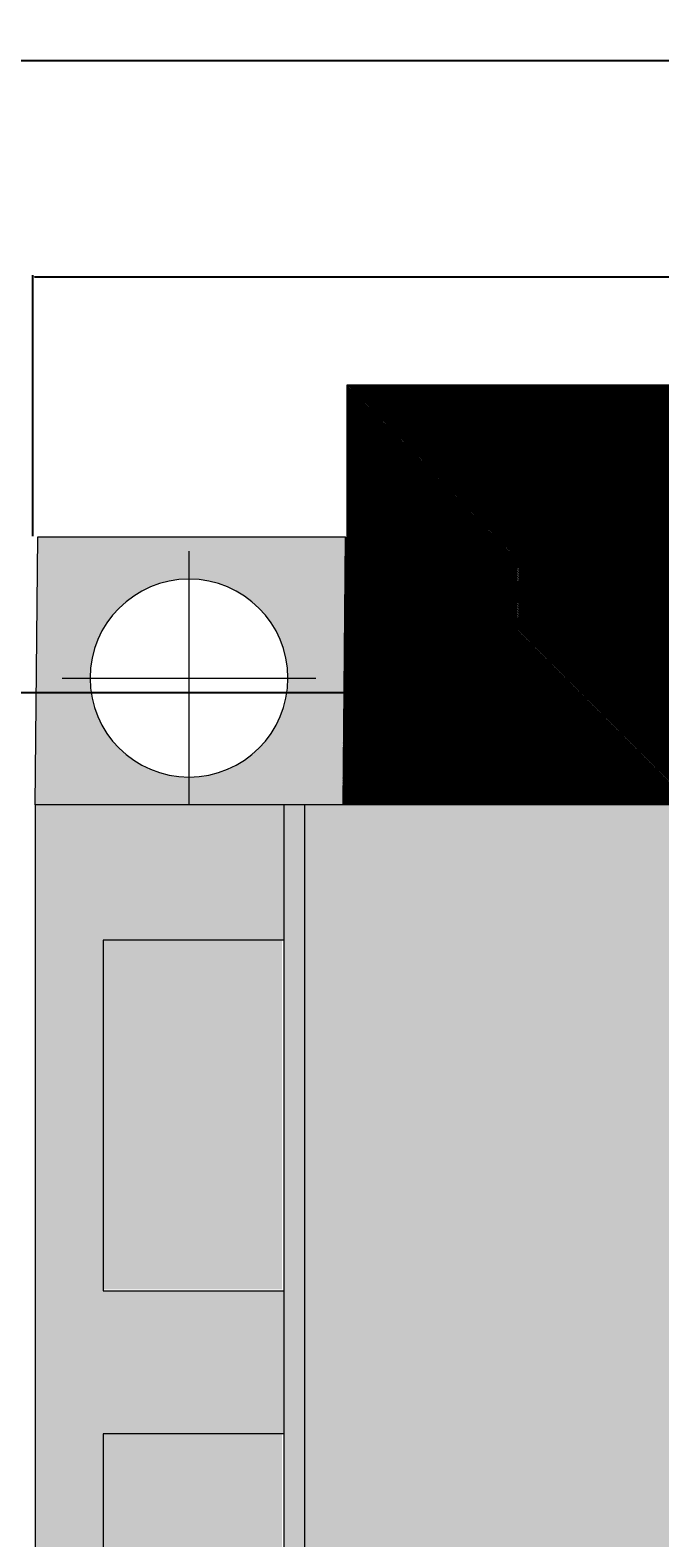
# Model space of a CAD drawing. Units: inches. Extents: x 192 to 1361, y -1362 to 367.
# Tile 7 of 23: x 293 to 361, y -616 to -454. Entities that reach past the tile are written whole.
import ezdxf

# ---------------------------------------------------------------- set-up
doc = ezdxf.new("R2010")
doc.units = ezdxf.units.IN
doc.header["$MEASUREMENT"] = 0
for name, color, linetype, lineweight in [('A-ANNO-DIMS', 2, 'Continuous', 18), ('A-FLOR', 8, 'Continuous', 18), ('furniture', 32, 'Continuous', 18)]:
    doc.layers.add(name, color=color, linetype=linetype, lineweight=lineweight)
doc.layers.add('A-FLOR-PATT', color=254, linetype='Continuous', lineweight=13, true_color=0xfeeab9)
doc.layers.add('A-FURN-PATT', color=254, linetype='Continuous', lineweight=13, true_color=0xfeeab9)
doc.styles.get("Standard").update_dxf_attribs({"font": 'arial.ttf'})
doc.dimstyles.get("Standard").update_dxf_attribs({"dimtxt": 0.18, "dimasz": 0.18, "dimexe": 0.18, "dimexo": 0.0625, "dimgap": 0.09, "dimtad": 0, "dimtih": 1, "dimtoh": 1, "dimzin": 0, "dimdsep": 46, "dimlunit": 3, "dimtxsty": 'Standard', "dimcen": 0.09, "dimadec": 0, "dimazin": 0, "dimtfac": 1, "dimtofl": 0, "dimtmove": 0, "dimatfit": 3, "dimfxl": 1, "dimtolj": 1, "dimtzin": 0, "dimarcsym": 0})

# ---------------------------------------------------------------- blocks, each defined once
blk = doc.blocks.new('A$C58D270C6')
at = {"layer": 'furniture'}
for p, q in [((14.974, 94.844), (14.974, 36)), ((16.217, 94.932), (16.217, 36)), ((9.25, 36), (9.25, 20.738)), ((1.618, 28.369), (16.881, 28.369))]:
    blk.add_line(p, q, dxfattribs=at)
for points in [[(0, 108), (77.905, 108), (77.905, 36), (0, 36)], [(4.094, 94.932), (14.974, 94.932), (14.974, 73.835), (4.094, 73.835)], [(4.094, 65.227), (14.974, 65.227), (14.974, 44.13), (4.094, 44.13)], [(18.655, 19.869), (18.499, 36), (0, 36), (0.156, 19.869)]]:
    blk.add_lwpolyline(points, close=True, dxfattribs=at)
blk.add_circle((9.25, 28.369), 5.955, dxfattribs=at)
blk = doc.blocks.new('*D24')
at = {"layer": 'A-ANNO-DIMS', "color": 0, "lineweight": -2, "transparency": 16777216}
for p, q in [((293.48, -508.38), (293.48, -480.42)), ((293.66, -480.6), (378, -480.6)), ((462.89, -480.6), (378.56, -480.6)), ((463.07, -508.38), (463.07, -480.42))]:
    blk.add_line(p, q, dxfattribs=at)
at = {"layer": 'A-ANNO-DIMS', "color": 0, "transparency": 16777216}
for points in [[(293.66, -480.57), (293.66, -480.63), (293.48, -480.6)], [(462.89, -480.57), (462.89, -480.63), (463.07, -480.6)]]:
    blk.add_solid(points, dxfattribs=at)
at = {"layer": 'Defpoints', "color": 0, "transparency": 16777216}
for p in [(463.07, -480.6), (293.48, -508.44), (463.07, -508.44)]:
    blk.add_point(p, dxfattribs=at)
at = {"layer": 'A-ANNO-DIMS', "color": 0, "transparency": 16777216, "insert": (378.28, -480.6), "char_height": 0.18, "attachment_point": 5}
blk.add_mtext('\\A1;170', dxfattribs=at)
blk = doc.blocks.new('*D48')
at = {"layer": 'A-ANNO-DIMS', "color": 0, "lineweight": -2, "transparency": 16777216}
for p, q in [((325.63, 258.53), (192.16, 258.53)), ((192.34, 258.35), (192.34, -429.22)), ((192.34, -1117.14), (192.34, -429.58)), ((395.21, -1117.32), (192.16, -1117.32))]:
    blk.add_line(p, q, dxfattribs=at)
at = {"layer": 'A-ANNO-DIMS', "color": 0, "transparency": 16777216}
for points in [[(192.31, 258.35), (192.37, 258.35), (192.34, 258.53)], [(192.31, -1117.14), (192.37, -1117.14), (192.34, -1117.32)]]:
    blk.add_solid(points, dxfattribs=at)
at = {"layer": 'Defpoints', "color": 0, "transparency": 16777216}
for p in [(325.7, 258.53), (192.34, -1117.32), (395.28, -1117.32)]:
    blk.add_point(p, dxfattribs=at)
at = {"layer": 'A-ANNO-DIMS', "color": 0, "transparency": 16777216, "insert": (192.34, -429.4), "char_height": 0.18, "attachment_point": 5}
blk.add_mtext('\\A1;1375.9', dxfattribs=at)
blk = doc.blocks.new('*D69')
at = {"layer": 'A-ANNO-DIMS', "color": 0, "lineweight": -2, "transparency": 16777216}
for p, q in [((981.75, -457.5), (192.16, -457.5)), ((192.34, -457.68), (192.34, -491.13)), ((192.34, -524.95), (192.34, -491.5)), ((980.52, -525.13), (192.16, -525.13))]:
    blk.add_line(p, q, dxfattribs=at)
at = {"layer": 'A-ANNO-DIMS', "color": 0, "transparency": 16777216}
for points in [[(192.31, -457.68), (192.37, -457.68), (192.34, -457.5)], [(192.31, -524.95), (192.37, -524.95), (192.34, -525.13)]]:
    blk.add_solid(points, dxfattribs=at)
at = {"layer": 'Defpoints', "color": 0, "transparency": 16777216}
for p in [(981.81, -457.5), (192.34, -525.13), (980.58, -525.13)]:
    blk.add_point(p, dxfattribs=at)
at = {"layer": 'A-ANNO-DIMS', "color": 0, "transparency": 16777216, "insert": (192.34, -491.31), "char_height": 0.18, "attachment_point": 5}
blk.add_mtext('\\A1;67.63', dxfattribs=at)

msp = doc.modelspace()

# ---------------------------------------------------------------- hatches: boundary and pattern name
at = {"layer": 'A-FLOR-PATT'}
h = msp.add_hatch(dxfattribs=at)
h.set_pattern_fill('ANSI31', color=256)
edge = h.paths.add_edge_path()
edge.add_line((513.1511, -492.1899), (327.1032, -492.1899))
edge.add_line((327.1032, -492.1899), (327.1032, -508.439))
edge.add_line((327.1032, -508.439), (326.9465, -508.439))
edge.add_line((326.9465, -508.439), (326.6697, -537.1419))
edge.add_line((326.6697, -537.1419), (391.8439, -537.1419))
edge.add_line((391.8439, -537.1419), (391.8439, -520.2026))
edge.add_line((391.8439, -520.2026), (393.0084, -520.2026))
edge.add_spline(control_points=[(393.2858, -517.1545), (392.9584, -517.4172), (392.3119, -517.936), (392.9583, -518.8629), (393.4257, -519.6151), (393.1386, -520.0192), (393.0084, -520.2026)], knot_values=[0, 0, 0, 0, 0.65327829, 1.2901376, 1.74045698, 2.11445126, 2.11445126, 2.11445126, 2.11445126], degree=3, periodic=0)
edge.add_line((393.0084, -520.2026), (395.1098, -520.2026))
edge.add_spline(control_points=[(395.3872, -517.1545), (395.0598, -517.4172), (394.4133, -517.936), (395.0598, -518.8629), (395.5272, -519.6151), (395.2401, -520.0192), (395.1098, -520.2026)], knot_values=[0, 0, 0, 0, 0.65327829, 1.2901376, 1.74045698, 2.11445126, 2.11445126, 2.11445126, 2.11445126], degree=3, periodic=0)
edge.add_line((395.1098, -520.2026), (397.3144, -520.2026))
edge.add_spline(control_points=[(397.5918, -517.1545), (397.2644, -517.4172), (396.6179, -517.936), (397.2643, -518.8629), (397.7317, -519.6151), (397.4446, -520.0192), (397.3144, -520.2026)], knot_values=[0, 0, 0, 0, 0.65327829, 1.2901376, 1.74045698, 2.11445126, 2.11445126, 2.11445126, 2.11445126], degree=3, periodic=0)
edge.add_line((397.3144, -520.2026), (399.2806, -520.2026))
edge.add_spline(control_points=[(399.558, -517.1545), (399.2307, -517.4172), (398.5841, -517.936), (399.2306, -518.8629), (399.698, -519.6151), (399.4109, -520.0192), (399.2806, -520.2026)], knot_values=[0, 0, 0, 0, 0.65327829, 1.2901376, 1.74045698, 2.11445126, 2.11445126, 2.11445126, 2.11445126], degree=3, periodic=0)
edge.add_line((399.2806, -520.2026), (401.664, -520.2026))
edge.add_spline(control_points=[(401.9414, -517.1545), (401.614, -517.4172), (400.9675, -517.936), (401.6139, -518.8629), (402.0814, -519.6151), (401.7943, -520.0192), (401.664, -520.2026)], knot_values=[0, 0, 0, 0, 0.65327829, 1.2901376, 1.74045698, 2.11445126, 2.11445126, 2.11445126, 2.11445126], degree=3, periodic=0)
edge.add_line((401.664, -520.2026), (403.6961, -520.2026))
edge.add_spline(control_points=[(403.9735, -517.1545), (403.6461, -517.4172), (402.9996, -517.936), (403.6461, -518.8629), (404.1135, -519.6151), (403.8264, -520.0192), (403.6961, -520.2026)], knot_values=[0, 0, 0, 0, 0.65327829, 1.2901376, 1.74045698, 2.11445126, 2.11445126, 2.11445126, 2.11445126], degree=3, periodic=0)
edge.add_line((403.6961, -520.2026), (405.6624, -520.2026))
edge.add_spline(control_points=[(405.9398, -517.1545), (405.6124, -517.4172), (404.9659, -517.936), (405.6123, -518.8629), (406.0797, -519.6151), (405.7926, -520.0192), (405.6624, -520.2026)], knot_values=[0, 0, 0, 0, 0.65327829, 1.2901376, 1.74045698, 2.11445126, 2.11445126, 2.11445126, 2.11445126], degree=3, periodic=0)
edge.add_line((405.6624, -520.2026), (408.0457, -520.2026))
edge.add_spline(control_points=[(408.3231, -517.1545), (407.9958, -517.4172), (407.3493, -517.936), (407.9957, -518.8629), (408.4631, -519.6151), (408.176, -520.0192), (408.0457, -520.2026)], knot_values=[0, 0, 0, 0, 0.65327829, 1.2901376, 1.74045698, 2.11445126, 2.11445126, 2.11445126, 2.11445126], degree=3, periodic=0)
edge.add_line((408.0457, -520.2026), (410.8462, -520.2026))
edge.add_spline(control_points=[(411.1236, -517.1545), (410.7962, -517.4172), (410.1497, -517.936), (410.7961, -518.8629), (411.2635, -519.6151), (410.9764, -520.0192), (410.8462, -520.2026)], knot_values=[0, 0, 0, 0, 0.65327829, 1.2901376, 1.74045698, 2.11445126, 2.11445126, 2.11445126, 2.11445126], degree=3, periodic=0)
edge.add_line((410.8462, -520.2026), (413.2295, -520.2026))
edge.add_spline(control_points=[(413.5069, -517.1545), (413.1795, -517.4172), (412.533, -517.936), (413.1794, -518.8629), (413.6468, -519.6151), (413.3597, -520.0192), (413.2295, -520.2026)], knot_values=[0, 0, 0, 0, 0.65327829, 1.2901376, 1.74045698, 2.11445126, 2.11445126, 2.11445126, 2.11445126], degree=3, periodic=0)
edge.add_line((413.2295, -520.2026), (415.434, -520.2026))
edge.add_spline(control_points=[(415.7114, -517.1545), (415.3841, -517.4172), (414.7376, -517.936), (415.384, -518.8629), (415.8514, -519.6151), (415.5643, -520.0192), (415.434, -520.2026)], knot_values=[0, 0, 0, 0, 0.65327829, 1.2901376, 1.74045698, 2.11445126, 2.11445126, 2.11445126, 2.11445126], degree=3, periodic=0)
edge.add_line((415.434, -520.2026), (417.5321, -520.2026))
edge.add_spline(control_points=[(417.8095, -517.1545), (417.4821, -517.4172), (416.8356, -517.936), (417.482, -518.8629), (417.9494, -519.6151), (417.6623, -520.0192), (417.5321, -520.2026)], knot_values=[0, 0, 0, 0, 0.65327829, 1.2901376, 1.74045698, 2.11445126, 2.11445126, 2.11445126, 2.11445126], degree=3, periodic=0)
edge.add_line((417.5321, -520.2026), (419.7366, -520.2026))
edge.add_spline(control_points=[(420.014, -517.1545), (419.6867, -517.4172), (419.0401, -517.936), (419.6866, -518.8629), (420.154, -519.6151), (419.8669, -520.0192), (419.7366, -520.2026)], knot_values=[0, 0, 0, 0, 0.65327829, 1.2901376, 1.74045698, 2.11445126, 2.11445126, 2.11445126, 2.11445126], degree=3, periodic=0)
edge.add_line((419.7366, -520.2026), (421.7029, -520.2026))
edge.add_spline(control_points=[(421.9803, -517.1545), (421.6529, -517.4172), (421.0064, -517.936), (421.6528, -518.8629), (422.1202, -519.6151), (421.8331, -520.0192), (421.7029, -520.2026)], knot_values=[0, 0, 0, 0, 0.65327829, 1.2901376, 1.74045698, 2.11445126, 2.11445126, 2.11445126, 2.11445126], degree=3, periodic=0)
edge.add_line((421.7029, -520.2026), (424.0863, -520.2026))
edge.add_spline(control_points=[(424.3637, -517.1545), (424.0363, -517.4172), (423.3898, -517.936), (424.0362, -518.8629), (424.5036, -519.6151), (424.2165, -520.0192), (424.0863, -520.2026)], knot_values=[0, 0, 0, 0, 0.65327829, 1.2901376, 1.74045698, 2.11445126, 2.11445126, 2.11445126, 2.11445126], degree=3, periodic=0)
edge.add_line((424.0863, -520.2026), (426.1184, -520.2026))
edge.add_spline(control_points=[(426.3958, -517.1545), (426.0684, -517.4172), (425.4219, -517.936), (426.0683, -518.8629), (426.5357, -519.6151), (426.2486, -520.0192), (426.1184, -520.2026)], knot_values=[0, 0, 0, 0, 0.65327829, 1.2901376, 1.74045698, 2.11445126, 2.11445126, 2.11445126, 2.11445126], degree=3, periodic=0)
edge.add_line((426.1184, -520.2026), (428.0846, -520.2026))
edge.add_spline(control_points=[(428.362, -517.1545), (428.0346, -517.4172), (427.3881, -517.936), (428.0346, -518.8629), (428.502, -519.6151), (428.2149, -520.0192), (428.0846, -520.2026)], knot_values=[0, 0, 0, 0, 0.65327829, 1.2901376, 1.74045698, 2.11445126, 2.11445126, 2.11445126, 2.11445126], degree=3, periodic=0)
edge.add_line((428.0846, -520.2026), (430.468, -520.2026))
edge.add_spline(control_points=[(430.7454, -517.1545), (430.418, -517.4172), (429.7715, -517.936), (430.4179, -518.8629), (430.8853, -519.6151), (430.5983, -520.0192), (430.468, -520.2026)], knot_values=[0, 0, 0, 0, 0.65327829, 1.2901376, 1.74045698, 2.11445126, 2.11445126, 2.11445126, 2.11445126], degree=3, periodic=0)
edge.add_line((430.468, -520.2026), (433.2684, -520.2026))
edge.add_spline(control_points=[(433.5458, -517.1545), (433.2184, -517.4172), (432.5719, -517.936), (433.2184, -518.8629), (433.6858, -519.6151), (433.3987, -520.0192), (433.2684, -520.2026)], knot_values=[0, 0, 0, 0, 0.65327829, 1.2901376, 1.74045698, 2.11445126, 2.11445126, 2.11445126, 2.11445126], degree=3, periodic=0)
edge.add_line((433.2684, -520.2026), (435.6517, -520.2026))
edge.add_spline(control_points=[(435.9291, -517.1545), (435.6017, -517.4172), (434.9552, -517.936), (435.6017, -518.8629), (436.0691, -519.6151), (435.782, -520.0192), (435.6517, -520.2026)], knot_values=[0, 0, 0, 0, 0.65327829, 1.2901376, 1.74045698, 2.11445126, 2.11445126, 2.11445126, 2.11445126], degree=3, periodic=0)
edge.add_line((435.6517, -520.2026), (437.8563, -520.2026))
edge.add_spline(control_points=[(438.1337, -517.1545), (437.8063, -517.4172), (437.1598, -517.936), (437.8062, -518.8629), (438.2736, -519.6151), (437.9865, -520.0192), (437.8563, -520.2026)], knot_values=[0, 0, 0, 0, 0.65327829, 1.2901376, 1.74045698, 2.11445126, 2.11445126, 2.11445126, 2.11445126], degree=3, periodic=0)
edge.add_line((437.8563, -520.2026), (439.7189, -520.2026))
edge.add_spline(control_points=[(439.9963, -517.1545), (439.669, -517.4172), (439.0225, -517.936), (439.6689, -518.8629), (440.1363, -519.6151), (439.8492, -520.0192), (439.7189, -520.2026)], knot_values=[0, 0, 0, 0, 0.65327829, 1.2901376, 1.74045698, 2.11445126, 2.11445126, 2.11445126, 2.11445126], degree=3, periodic=0)
edge.add_line((439.7189, -520.2026), (441.9235, -520.2026))
edge.add_spline(control_points=[(442.2009, -517.1545), (441.8735, -517.4172), (441.227, -517.936), (441.8735, -518.8629), (442.3409, -519.6151), (442.0538, -520.0192), (441.9235, -520.2026)], knot_values=[0, 0, 0, 0, 0.65327829, 1.2901376, 1.74045698, 2.11445126, 2.11445126, 2.11445126, 2.11445126], degree=3, periodic=0)
edge.add_line((441.9235, -520.2026), (443.8898, -520.2026))
edge.add_spline(control_points=[(444.1672, -517.1545), (443.8398, -517.4172), (443.1933, -517.936), (443.8397, -518.8629), (444.3071, -519.6151), (444.02, -520.0192), (443.8898, -520.2026)], knot_values=[0, 0, 0, 0, 0.65327829, 1.2901376, 1.74045698, 2.11445126, 2.11445126, 2.11445126, 2.11445126], degree=3, periodic=0)
edge.add_line((443.8898, -520.2026), (446.2731, -520.2026))
edge.add_spline(control_points=[(446.5505, -517.1545), (446.2232, -517.4172), (445.5767, -517.936), (446.2231, -518.8629), (446.6905, -519.6151), (446.4034, -520.0192), (446.2731, -520.2026)], knot_values=[0, 0, 0, 0, 0.65327829, 1.2901376, 1.74045698, 2.11445126, 2.11445126, 2.11445126, 2.11445126], degree=3, periodic=0)
edge.add_line((446.2731, -520.2026), (448.3052, -520.2026))
edge.add_spline(control_points=[(448.5826, -517.1545), (448.2553, -517.4172), (447.6088, -517.936), (448.2552, -518.8629), (448.7226, -519.6151), (448.4355, -520.0192), (448.3052, -520.2026)], knot_values=[0, 0, 0, 0, 0.65327829, 1.2901376, 1.74045698, 2.11445126, 2.11445126, 2.11445126, 2.11445126], degree=3, periodic=0)
edge.add_line((448.3052, -520.2026), (450.2715, -520.2026))
edge.add_spline(control_points=[(450.5489, -517.1545), (450.2215, -517.4172), (449.575, -517.936), (450.2214, -518.8629), (450.6888, -519.6151), (450.4018, -520.0192), (450.2715, -520.2026)], knot_values=[0, 0, 0, 0, 0.65327829, 1.2901376, 1.74045698, 2.11445126, 2.11445126, 2.11445126, 2.11445126], degree=3, periodic=0)
edge.add_line((450.2715, -520.2026), (452.6549, -520.2026))
edge.add_spline(control_points=[(452.9323, -517.1545), (452.6049, -517.4172), (451.9584, -517.936), (452.6048, -518.8629), (453.0722, -519.6151), (452.7851, -520.0192), (452.6549, -520.2026)], knot_values=[0, 0, 0, 0, 0.65327829, 1.2901376, 1.74045698, 2.11445126, 2.11445126, 2.11445126, 2.11445126], degree=3, periodic=0)
edge.add_line((452.6549, -520.2026), (453.8151, -520.2026))
edge.add_spline(control_points=[(454.0925, -517.1545), (453.7499, -517.417), (453.0754, -517.9338), (453.769, -518.8576), (454.2314, -519.6154), (453.945, -520.0193), (453.8151, -520.2026)], knot_values=[0, 0, 0, 0, 0.6639037, 1.30740562, 1.757725, 2.13171928, 2.13171928, 2.13171928, 2.13171928], degree=3, periodic=0)
edge.add_line((453.8151, -520.2026), (455.3467, -520.2026))
edge.add_spline(control_points=[(455.6241, -517.1545), (455.2967, -517.4172), (454.6502, -517.936), (455.2967, -518.8629), (455.7641, -519.6151), (455.477, -520.0192), (455.3467, -520.2026)], knot_values=[0, 0, 0, 0, 0.65327829, 1.2901376, 1.74045698, 2.11445126, 2.11445126, 2.11445126, 2.11445126], degree=3, periodic=0)
edge.add_line((455.3467, -520.2026), (456.895, -520.2026))
edge.add_spline(control_points=[(456.895, -520.2026), (457.0253, -520.0192), (457.3124, -519.6151), (456.845, -518.8629), (456.1986, -517.936), (456.8451, -517.4172), (457.1724, -517.1545)], knot_values=[0, 0, 0, 0, 0.37399428, 0.82431366, 1.46117297, 2.11445126, 2.11445126, 2.11445126, 2.11445126], degree=3, periodic=0)
edge.add_spline(control_points=[(458.0074, -517.1545), (457.68, -517.4172), (457.0335, -517.936), (457.68, -518.8629), (458.1474, -519.6151), (457.8603, -520.0192), (457.73, -520.2026)], knot_values=[0, 0, 0, 0, 0.65327829, 1.2901376, 1.74045698, 2.11445126, 2.11445126, 2.11445126, 2.11445126], degree=3, periodic=0)
edge.add_line((457.73, -520.2026), (458.8613, -520.2026))
edge.add_spline(control_points=[(459.1387, -517.1545), (458.8113, -517.4172), (458.1648, -517.936), (458.8112, -518.8629), (459.2786, -519.6151), (458.9916, -520.0192), (458.8613, -520.2026)], knot_values=[0, 0, 0, 0, 0.65327829, 1.2901376, 1.74045698, 2.11445126, 2.11445126, 2.11445126, 2.11445126], degree=3, periodic=0)
edge.add_line((458.8613, -520.2026), (459.9346, -520.2026))
edge.add_spline(control_points=[(460.212, -517.1545), (459.8846, -517.4172), (459.2381, -517.936), (459.8845, -518.8629), (460.3519, -519.6151), (460.0648, -520.0192), (459.9346, -520.2026)], knot_values=[0, 0, 0, 0, 0.65327829, 1.2901376, 1.74045698, 2.11445126, 2.11445126, 2.11445126, 2.11445126], degree=3, periodic=0)
edge.add_line((459.9346, -520.2026), (461.2447, -520.2026))
edge.add_spline(control_points=[(461.5221, -517.1545), (461.1947, -517.4172), (460.5482, -517.936), (461.1946, -518.8629), (461.662, -519.6151), (461.3749, -520.0192), (461.2447, -520.2026)], knot_values=[0, 0, 0, 0, 0.65327829, 1.2901376, 1.74045698, 2.11445126, 2.11445126, 2.11445126, 2.11445126], degree=3, periodic=0)
edge.add_line((461.2447, -520.2026), (462.6002, -520.2026))
edge.add_spline(control_points=[(462.8776, -517.1545), (462.5502, -517.4172), (461.9037, -517.936), (462.5501, -518.8629), (463.0175, -519.6151), (462.7304, -520.0192), (462.6002, -520.2026)], knot_values=[0, 0, 0, 0, 0.65327829, 1.2901376, 1.74045698, 2.11445126, 2.11445126, 2.11445126, 2.11445126], degree=3, periodic=0)
edge.add_line((462.6002, -520.2026), (463.0739, -520.2026))
edge.add_line((463.0739, -520.2026), (463.0739, -691.0271))
edge.add_line((463.0739, -691.0271), (462.6214, -691.0271))
edge.add_spline(control_points=[(462.8776, -694.0453), (462.5502, -693.7826), (461.9037, -693.2638), (462.5501, -692.3369), (463.011, -691.5951), (462.7443, -691.2005), (462.6214, -691.0271)], knot_values=[0, 0, 0, 0, 0.65327829, 1.2901376, 1.74045698, 2.09412198, 2.09412198, 2.09412198, 2.09412198], degree=3, periodic=0)
edge.add_line((462.6214, -691.0271), (461.3416, -691.0271))
edge.add_spline(control_points=[(461.5978, -694.0453), (461.2704, -693.7826), (460.6239, -693.2638), (461.2703, -692.3369), (461.7312, -691.5951), (461.4644, -691.2005), (461.3416, -691.0271)], knot_values=[0, 0, 0, 0, 0.65327829, 1.2901376, 1.74045698, 2.09412198, 2.09412198, 2.09412198, 2.09412198], degree=3, periodic=0)
edge.add_line((461.3416, -691.0271), (460.0315, -691.0271))
edge.add_spline(control_points=[(460.2877, -694.0453), (459.9603, -693.7826), (459.3138, -693.2638), (459.9602, -692.3369), (460.4211, -691.5951), (460.1544, -691.2005), (460.0315, -691.0271)], knot_values=[0, 0, 0, 0, 0.65327829, 1.2901376, 1.74045698, 2.09412198, 2.09412198, 2.09412198, 2.09412198], degree=3, periodic=0)
edge.add_line((460.0315, -691.0271), (458.9582, -691.0271))
edge.add_spline(control_points=[(459.2144, -694.0453), (458.887, -693.7826), (458.2405, -693.2638), (458.8869, -692.3369), (459.3478, -691.5951), (459.0811, -691.2005), (458.9582, -691.0271)], knot_values=[0, 0, 0, 0, 0.65327829, 1.2901376, 1.74045698, 2.09412198, 2.09412198, 2.09412198, 2.09412198], degree=3, periodic=0)
edge.add_line((458.9582, -691.0271), (457.8269, -691.0271))
edge.add_spline(control_points=[(457.8269, -691.0271), (457.9464, -691.2008), (458.2187, -691.5966), (457.7545, -692.3366), (457.1096, -693.2638), (457.7558, -693.7826), (458.0831, -694.0453)], knot_values=[0, 0, 0, 0, 0.3521435, 0.80246288, 1.43932219, 2.09260048, 2.09260048, 2.09260048, 2.09260048], degree=3, periodic=0)
edge.add_spline(control_points=[(457.2481, -694.0453), (456.9209, -693.7826), (456.2746, -693.2638), (456.9195, -692.3366), (457.3837, -691.5966), (457.1114, -691.2008), (456.992, -691.0271)], knot_values=[0, 0, 0, 0, 0.65327829, 1.2901376, 1.74045698, 2.09260048, 2.09260048, 2.09260048, 2.09260048], degree=3, periodic=0)
edge.add_line((456.992, -691.0271), (455.4436, -691.0271))
edge.add_spline(control_points=[(455.6998, -694.0453), (455.3725, -693.7826), (454.7263, -693.2638), (455.3712, -692.3366), (455.8354, -691.5966), (455.5631, -691.2008), (455.4436, -691.0271)], knot_values=[0, 0, 0, 0, 0.65327829, 1.2901376, 1.74045698, 2.09260048, 2.09260048, 2.09260048, 2.09260048], degree=3, periodic=0)
edge.add_line((455.4436, -691.0271), (453.8363, -691.0271))
edge.add_spline(control_points=[(454.0925, -694.0453), (453.7602, -693.7827), (453.1046, -693.2646), (453.7653, -692.3383), (454.2277, -691.5965), (453.9557, -691.2008), (453.8363, -691.0271)], knot_values=[0, 0, 0, 0, 0.65679228, 1.29582582, 1.7461452, 2.0982924, 2.0982924, 2.0982924, 2.0982924], degree=3, periodic=0)
edge.add_line((453.8363, -691.0271), (452.6761, -691.0271))
edge.add_spline(control_points=[(452.9323, -694.0453), (452.605, -693.7826), (451.9587, -693.2638), (452.6037, -692.3366), (453.0678, -691.5966), (452.7956, -691.2008), (452.6761, -691.0271)], knot_values=[0, 0, 0, 0, 0.65327829, 1.2901376, 1.74045698, 2.09260048, 2.09260048, 2.09260048, 2.09260048], degree=3, periodic=0)
edge.add_line((452.6761, -691.0271), (450.2927, -691.0271))
edge.add_spline(control_points=[(450.5489, -694.0453), (450.2216, -693.7826), (449.5753, -693.2638), (450.2203, -692.3366), (450.6845, -691.5966), (450.4122, -691.2008), (450.2927, -691.0271)], knot_values=[0, 0, 0, 0, 0.65327829, 1.2901376, 1.74045698, 2.09260048, 2.09260048, 2.09260048, 2.09260048], degree=3, periodic=0)
edge.add_line((450.2927, -691.0271), (448.3265, -691.0271))
edge.add_spline(control_points=[(448.5826, -694.0453), (448.2553, -693.7826), (447.6088, -693.2638), (448.2552, -692.3369), (448.7161, -691.5951), (448.4493, -691.2005), (448.3265, -691.0271)], knot_values=[0, 0, 0, 0, 0.65327829, 1.2901376, 1.74045698, 2.09412198, 2.09412198, 2.09412198, 2.09412198], degree=3, periodic=0)
edge.add_line((448.3265, -691.0271), (446.2944, -691.0271))
edge.add_spline(control_points=[(446.5505, -694.0453), (446.2232, -693.7826), (445.5767, -693.2638), (446.2231, -692.3369), (446.684, -691.5951), (446.4172, -691.2005), (446.2944, -691.0271)], knot_values=[0, 0, 0, 0, 0.65327829, 1.2901376, 1.74045698, 2.09412198, 2.09412198, 2.09412198, 2.09412198], degree=3, periodic=0)
edge.add_line((446.2944, -691.0271), (443.911, -691.0271))
edge.add_spline(control_points=[(444.1672, -694.0453), (443.8398, -693.7826), (443.1933, -693.2638), (443.8397, -692.3369), (444.3006, -691.5951), (444.0338, -691.2005), (443.911, -691.0271)], knot_values=[0, 0, 0, 0, 0.65327829, 1.2901376, 1.74045698, 2.09412198, 2.09412198, 2.09412198, 2.09412198], degree=3, periodic=0)
edge.add_line((443.911, -691.0271), (441.9447, -691.0271))
edge.add_spline(control_points=[(442.2009, -694.0453), (441.8735, -693.7826), (441.227, -693.2638), (441.8735, -692.3369), (442.3344, -691.5951), (442.0676, -691.2005), (441.9447, -691.0271)], knot_values=[0, 0, 0, 0, 0.65327829, 1.2901376, 1.74045698, 2.09412198, 2.09412198, 2.09412198, 2.09412198], degree=3, periodic=0)
edge.add_line((441.9447, -691.0271), (439.7402, -691.0271))
edge.add_spline(control_points=[(439.9963, -694.0453), (439.669, -693.7826), (439.0225, -693.2638), (439.6689, -692.3369), (440.1298, -691.5951), (439.863, -691.2005), (439.7402, -691.0271)], knot_values=[0, 0, 0, 0, 0.65327829, 1.2901376, 1.74045698, 2.09412198, 2.09412198, 2.09412198, 2.09412198], degree=3, periodic=0)
edge.add_line((439.7402, -691.0271), (437.8775, -691.0271))
edge.add_spline(control_points=[(438.1337, -694.0453), (437.8063, -693.7826), (437.1598, -693.2638), (437.8062, -692.3369), (438.2671, -691.5951), (438.0004, -691.2005), (437.8775, -691.0271)], knot_values=[0, 0, 0, 0, 0.65327829, 1.2901376, 1.74045698, 2.09412198, 2.09412198, 2.09412198, 2.09412198], degree=3, periodic=0)
edge.add_line((437.8775, -691.0271), (435.6729, -691.0271))
edge.add_spline(control_points=[(435.9291, -694.0453), (435.6017, -693.7826), (434.9552, -693.2638), (435.6017, -692.3369), (436.0626, -691.5951), (435.7958, -691.2005), (435.6729, -691.0271)], knot_values=[0, 0, 0, 0, 0.65327829, 1.2901376, 1.74045698, 2.09412198, 2.09412198, 2.09412198, 2.09412198], degree=3, periodic=0)
edge.add_line((435.6729, -691.0271), (433.2896, -691.0271))
edge.add_spline(control_points=[(433.5458, -694.0453), (433.2184, -693.7826), (432.5719, -693.2638), (433.2184, -692.3369), (433.6793, -691.5951), (433.4125, -691.2005), (433.2896, -691.0271)], knot_values=[0, 0, 0, 0, 0.65327829, 1.2901376, 1.74045698, 2.09412198, 2.09412198, 2.09412198, 2.09412198], degree=3, periodic=0)
edge.add_line((433.2896, -691.0271), (430.4892, -691.0271))
edge.add_spline(control_points=[(430.7454, -694.0453), (430.418, -693.7826), (429.7715, -693.2638), (430.4179, -692.3369), (430.8788, -691.5951), (430.6121, -691.2005), (430.4892, -691.0271)], knot_values=[0, 0, 0, 0, 0.65327829, 1.2901376, 1.74045698, 2.09412198, 2.09412198, 2.09412198, 2.09412198], degree=3, periodic=0)
edge.add_line((430.4892, -691.0271), (428.1058, -691.0271))
edge.add_spline(control_points=[(428.362, -694.0453), (428.0346, -693.7826), (427.3881, -693.2638), (428.0346, -692.3369), (428.4955, -691.5951), (428.2287, -691.2005), (428.1058, -691.0271)], knot_values=[0, 0, 0, 0, 0.65327829, 1.2901376, 1.74045698, 2.09412198, 2.09412198, 2.09412198, 2.09412198], degree=3, periodic=0)
edge.add_line((428.1058, -691.0271), (426.1396, -691.0271))
edge.add_spline(control_points=[(426.3958, -694.0453), (426.0684, -693.7826), (425.4219, -693.2638), (426.0683, -692.3369), (426.5292, -691.5951), (426.2624, -691.2005), (426.1396, -691.0271)], knot_values=[0, 0, 0, 0, 0.65327829, 1.2901376, 1.74045698, 2.09412198, 2.09412198, 2.09412198, 2.09412198], degree=3, periodic=0)
edge.add_line((426.1396, -691.0271), (424.1075, -691.0271))
edge.add_spline(control_points=[(424.3637, -694.0453), (424.0363, -693.7826), (423.3898, -693.2638), (424.0362, -692.3369), (424.4971, -691.5951), (424.2303, -691.2005), (424.1075, -691.0271)], knot_values=[0, 0, 0, 0, 0.65327829, 1.2901376, 1.74045698, 2.09412198, 2.09412198, 2.09412198, 2.09412198], degree=3, periodic=0)
edge.add_line((424.1075, -691.0271), (421.7241, -691.0271))
edge.add_spline(control_points=[(421.9803, -694.0453), (421.6529, -693.7826), (421.0064, -693.2638), (421.6528, -692.3369), (422.1137, -691.5951), (421.847, -691.2005), (421.7241, -691.0271)], knot_values=[0, 0, 0, 0, 0.65327829, 1.2901376, 1.74045698, 2.09412198, 2.09412198, 2.09412198, 2.09412198], degree=3, periodic=0)
edge.add_line((421.7241, -691.0271), (419.7579, -691.0271))
edge.add_spline(control_points=[(420.014, -694.0453), (419.6867, -693.7826), (419.0401, -693.2638), (419.6866, -692.3369), (420.1475, -691.5951), (419.8807, -691.2005), (419.7579, -691.0271)], knot_values=[0, 0, 0, 0, 0.65327829, 1.2901376, 1.74045698, 2.09412198, 2.09412198, 2.09412198, 2.09412198], degree=3, periodic=0)
edge.add_line((419.7579, -691.0271), (417.5533, -691.0271))
edge.add_spline(control_points=[(417.8095, -694.0453), (417.4821, -693.7826), (416.8356, -693.2638), (417.482, -692.3369), (417.9429, -691.5951), (417.6761, -691.2005), (417.5533, -691.0271)], knot_values=[0, 0, 0, 0, 0.65327829, 1.2901376, 1.74045698, 2.09412198, 2.09412198, 2.09412198, 2.09412198], degree=3, periodic=0)
edge.add_line((417.5533, -691.0271), (415.4553, -691.0271))
edge.add_spline(control_points=[(415.7114, -694.0453), (415.3841, -693.7826), (414.7376, -693.2638), (415.384, -692.3369), (415.8449, -691.5951), (415.5781, -691.2005), (415.4553, -691.0271)], knot_values=[0, 0, 0, 0, 0.65327829, 1.2901376, 1.74045698, 2.09412198, 2.09412198, 2.09412198, 2.09412198], degree=3, periodic=0)
edge.add_line((415.4553, -691.0271), (413.2507, -691.0271))
edge.add_spline(control_points=[(413.5069, -694.0453), (413.1795, -693.7826), (412.533, -693.2638), (413.1794, -692.3369), (413.6403, -691.5951), (413.3736, -691.2005), (413.2507, -691.0271)], knot_values=[0, 0, 0, 0, 0.65327829, 1.2901376, 1.74045698, 2.09412198, 2.09412198, 2.09412198, 2.09412198], degree=3, periodic=0)
edge.add_line((413.2507, -691.0271), (410.8674, -691.0271))
edge.add_spline(control_points=[(411.1236, -694.0453), (410.7962, -693.7826), (410.1497, -693.2638), (410.7961, -692.3369), (411.257, -691.5951), (410.9903, -691.2005), (410.8674, -691.0271)], knot_values=[0, 0, 0, 0, 0.65327829, 1.2901376, 1.74045698, 2.09412198, 2.09412198, 2.09412198, 2.09412198], degree=3, periodic=0)
edge.add_line((410.8674, -691.0271), (408.067, -691.0271))
edge.add_spline(control_points=[(408.3231, -694.0453), (407.9958, -693.7826), (407.3493, -693.2638), (407.9957, -692.3369), (408.4566, -691.5951), (408.1898, -691.2005), (408.067, -691.0271)], knot_values=[0, 0, 0, 0, 0.65327829, 1.2901376, 1.74045698, 2.09412198, 2.09412198, 2.09412198, 2.09412198], degree=3, periodic=0)
edge.add_line((408.067, -691.0271), (405.6836, -691.0271))
edge.add_spline(control_points=[(405.9398, -694.0453), (405.6124, -693.7826), (404.9659, -693.2638), (405.6123, -692.3369), (406.0732, -691.5951), (405.8064, -691.2005), (405.6836, -691.0271)], knot_values=[0, 0, 0, 0, 0.65327829, 1.2901376, 1.74045698, 2.09412198, 2.09412198, 2.09412198, 2.09412198], degree=3, periodic=0)
edge.add_line((405.6836, -691.0271), (403.7173, -691.0271))
edge.add_spline(control_points=[(403.9735, -694.0453), (403.6461, -693.7826), (402.9996, -693.2638), (403.6461, -692.3369), (404.107, -691.5951), (403.8402, -691.2005), (403.7173, -691.0271)], knot_values=[0, 0, 0, 0, 0.65327829, 1.2901376, 1.74045698, 2.09412198, 2.09412198, 2.09412198, 2.09412198], degree=3, periodic=0)
edge.add_line((403.7173, -691.0271), (401.6852, -691.0271))
edge.add_spline(control_points=[(401.9414, -694.0453), (401.614, -693.7826), (400.9675, -693.2638), (401.6139, -692.3369), (402.0749, -691.5951), (401.8081, -691.2005), (401.6852, -691.0271)], knot_values=[0, 0, 0, 0, 0.65327829, 1.2901376, 1.74045698, 2.09412198, 2.09412198, 2.09412198, 2.09412198], degree=3, periodic=0)
edge.add_line((401.6852, -691.0271), (399.3019, -691.0271))
edge.add_spline(control_points=[(399.558, -694.0453), (399.2307, -693.7826), (398.5841, -693.2638), (399.2306, -692.3369), (399.6915, -691.5951), (399.4247, -691.2005), (399.3019, -691.0271)], knot_values=[0, 0, 0, 0, 0.65327829, 1.2901376, 1.74045698, 2.09412198, 2.09412198, 2.09412198, 2.09412198], degree=3, periodic=0)
edge.add_line((399.3019, -691.0271), (397.3356, -691.0271))
edge.add_spline(control_points=[(397.5918, -694.0453), (397.2644, -693.7826), (396.6179, -693.2638), (397.2643, -692.3369), (397.7252, -691.5951), (397.4585, -691.2005), (397.3356, -691.0271)], knot_values=[0, 0, 0, 0, 0.65327829, 1.2901376, 1.74045698, 2.09412198, 2.09412198, 2.09412198, 2.09412198], degree=3, periodic=0)
edge.add_line((397.3356, -691.0271), (395.131, -691.0271))
edge.add_spline(control_points=[(395.3872, -694.0453), (395.0598, -693.7826), (394.4133, -693.2638), (395.0598, -692.3369), (395.5207, -691.5951), (395.2539, -691.2005), (395.131, -691.0271)], knot_values=[0, 0, 0, 0, 0.65327829, 1.2901376, 1.74045698, 2.09412198, 2.09412198, 2.09412198, 2.09412198], degree=3, periodic=0)
edge.add_line((395.131, -691.0271), (393.0296, -691.0271))
edge.add_spline(control_points=[(393.2858, -694.0453), (392.9584, -693.7826), (392.3119, -693.2638), (392.9583, -692.3369), (393.4192, -691.5951), (393.1524, -691.2005), (393.0296, -691.0271)], knot_values=[0, 0, 0, 0, 0.65327829, 1.2901376, 1.74045698, 2.09412198, 2.09412198, 2.09412198, 2.09412198], degree=3, periodic=0)
edge.add_line((393.0296, -691.0271), (391.8439, -691.0271))
edge.add_line((391.8439, -691.0271), (391.8439, -665.2551))
edge.add_line((391.8439, -665.2551), (326.6697, -665.2551))
edge.add_line((326.6697, -665.2551), (326.3929, -693.958))
edge.add_line((326.3929, -693.958), (326.3929, -716.9381))
edge.add_line((326.3929, -716.9381), (513.1511, -716.9381))
edge.add_line((513.1511, -716.9381), (513.1511, -492.1899))
h.paths.add_polyline_path([(353.9763, -588.1534), (487.3258, -588.1534), (487.3258, -561.3965), (353.9763, -561.3965)], flags=25)
at = {"layer": 'A-FURN-PATT'}
h = msp.add_hatch(color=256, dxfattribs=at)
h.dxf.hatch_style = 1
h.paths.add_polyline_path([(320.5124, -642.0022), (301.0388, -642.0022), (301.0388, -604.4633), (320.3977, -604.4633), (320.3977, -589.1472), (301.0388, -589.1472), (301.0388, -551.6082), (320.3977, -551.6082), (320.3977, -537.1419), (293.7534, -537.1419), (293.7534, -665.2551), (337.5553, -665.2551), (337.5553, -665.117)])
h.paths.add_polyline_path([(320.5305, -680.3795, -0.41421356), (309.9348, -690.9753), (309.9348, -693.958), (326.3929, -693.958), (326.6697, -665.2551), (293.7534, -665.2551), (293.4767, -693.958), (309.9348, -693.958), (309.9348, -690.9753, -0.41421356), (299.3391, -680.3795, -1)])
h.paths.add_polyline_path([(320.8073, -523.5634, -0.41421356), (310.2116, -534.1591), (310.2116, -537.1419), (326.6697, -537.1419), (326.9465, -508.439), (294.0302, -508.439), (293.7534, -537.1419), (310.2116, -537.1419), (310.2116, -534.1591, -0.41421356), (299.6159, -523.5634, -1)])
h = msp.add_hatch(color=256, dxfattribs=at)
h.dxf.hatch_style = 1
h.paths.add_polyline_path([(320.1552, -604.3144), (300.7962, -604.3144), (300.7962, -641.8533), (320.1552, -641.8533)])
h.paths.add_polyline_path([(320.1552, -551.4593), (300.7962, -551.4593), (300.7962, -588.9983), (320.1552, -588.9983)])
h.paths.add_polyline_path([(462.8313, -520.0537), (391.6014, -520.0537), (391.6014, -536.993), (432.1311, -536.993), (432.1311, -665.1062), (391.6014, -665.1062), (391.6014, -690.8782), (462.8313, -690.8782)])
h = msp.add_hatch(color=256, dxfattribs=at)
h.dxf.hatch_style = 1
h.paths.add_polyline_path([(337.5553, -642.0022), (320.5124, -642.0022), (337.5553, -665.117)])
h.paths.add_polyline_path([(322.6088, -537.1419), (320.3977, -537.1419), (320.3977, -641.8467), (320.5124, -642.0022), (322.6088, -642.0022)])
h = msp.add_hatch(color=256, dxfattribs=at)
h.dxf.hatch_style = 1
h.paths.add_polyline_path([(432.3737, -537.1419), (368.625, -537.1419), (368.625, -665.2551), (432.3737, -665.2551)])
h.paths.add_polyline_path([(368.625, -537.1419), (322.6088, -537.1419), (322.6088, -642.0022), (337.5553, -642.0022), (337.5553, -665.2551), (368.625, -665.2551)])

# ---------------------------------------------------------------- linework, layer by layer
at = {"layer": 'A-FLOR'}
for p, q in [((513.1511, -492.1899), (327.1032, -492.1899)), ((327.1032, -492.1899), (327.1032, -508.439))]:
    msp.add_line(p, q, dxfattribs=at)

# ---------------------------------------------------------------- block references
at = {"layer": 'furniture', "xscale": -1.779350280135438, "yscale": 1.779350280135438, "zscale": 1.779350280135438, "rotation": 180}
msp.add_blockref('A$C58D270C6', (293.7534, -473.0852), dxfattribs=at)

# ---------------------------------------------------------------- dimensions: what is measured, and where the dimension line sits
at = {"layer": 'A-ANNO-DIMS'}
for base, p1, p2, override, picture, middle in [((192.3425, -1117.3227), (325.6957, 258.5286), (395.2768, -1117.3227), {"dimdec": 1, "dimlfac": 1, "dimrnd": 0, "dimzin": 0, "dimdsep": 46, "dimlunit": 2}, '*D48', (192.3425, -429.3971)), ((192.3425, -525.128), (981.8078, -457.4996), (980.5799, -525.128), {"dimdec": 2, "dimlfac": 1, "dimrnd": 0, "dimzin": 0, "dimdsep": 46, "dimlunit": 2}, '*D69', (192.3425, -491.3138))]:
    dim = msp.add_linear_dim(base=base, p1=p1, p2=p2, angle=90, dimstyle='Standard', override=override, dxfattribs=at)
    dim.commit()
    dim.dimension.update_dxf_attribs({"geometry": picture, "text_midpoint": middle})
dim = msp.add_linear_dim(base=(463.0739, -480.598), p1=(293.4767, -508.439), p2=(463.0739, -508.439), dimstyle='Standard', override={"dimdec": 0, "dimlfac": 1, "dimrnd": 0, "dimzin": 0, "dimdsep": 46, "dimlunit": 2}, dxfattribs=at)
dim.commit()
dim.dimension.update_dxf_attribs({"geometry": '*D24', "text_midpoint": (378.2753, -480.598)})

doc.saveas('drawing.dxf')
